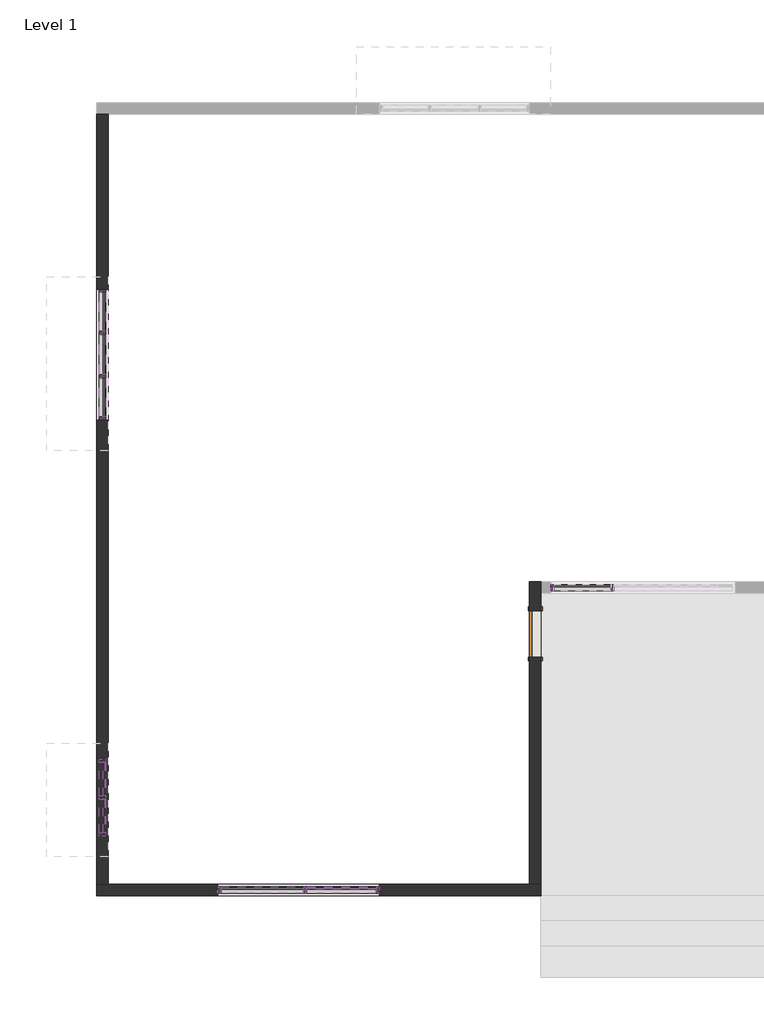
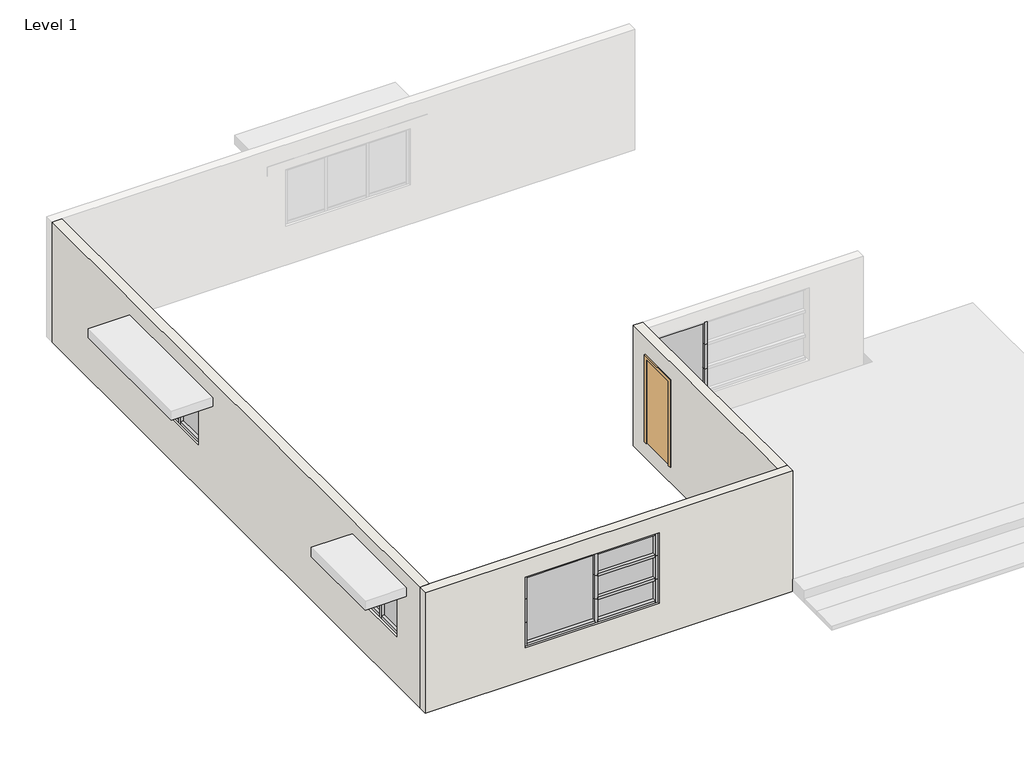
# One storey, part 1 of 2: 39 members, 10 plates, 3 walls, 1 door.
"""IFC4 building model written with IfcOpenShell, lengths in millimetres."""

from ifc_helpers import new_model, si_unit, frame, origin, place, context, project, spatial, polyline, outline, extrude, faceted_brep, transform, mapped, element, save
from components import door_0ca8825f, member_b864958b, member_e6b9f524, member_cfc9b631, member_58197c2e, member_50ab567a, member_249e519d, member_79cc3911, member_4dc7c44e, member_c33c434a, member_8ea09a22, member_05ffdb5f, member_d36207d9, member_46f5bc36, member_488afbc6, member_b07cc7a9, system_panel_glazed_a9ff3cf1, system_panel_glazed_35d8d551, system_panel_glazed_1724a70f, system_panel_glazed_43256be5, system_panel_glazed_960ffd39, system_panel_glazed_d0a3eec4, system_panel_glazed_ba533b82

model = new_model("IFC4")

# Units and contexts
model_context = context("Model", 3, world=origin())
ifc_project = project(units=[si_unit("LENGTHUNIT", "METRE", prefix="MILLI")], contexts=[model_context])

# Site, building, storey
site = spatial("IfcSite", under=ifc_project)
building = spatial("IfcBuilding", under=site)
storey = spatial("IfcBuildingStorey", under=building, Name="Level 1", Elevation=0.0)

# Door
placement = place(None, origin())
door_shape = door_0ca8825f(model_context)
element("IfcDoor", 1, ObjectType="Single-Flush : 36\" x 84\"", at=placement, inside=storey, context=model_context, shape_type="MappedRepresentation", body=[
    mapped(door_shape, transform((-11357.8120831, -6931.6945627, 406.4), x_axis=(0.0, 1.0, 0.0), y_axis=(-1.0, 0.0, 0.0), z_axis=(0.0, 0.0, 1.0))),
])

# Members
member_shape = member_b864958b(model_context)
element("IfcMember", 2, ObjectType="Rectangular Mullion : 2.5\" x 5\" rectangular", at=placement, inside=storey, context=model_context, shape_type="MappedRepresentation", body=[
    mapped(member_shape, transform((-11053.0120831, -6017.2945627, 2097.5096891), x_axis=(-1.0, 0.0, 0.0), y_axis=(0.0, -1.0, 0.0), z_axis=(0.0, 0.0, 1.0))),
])
element("IfcMember", 3, ObjectType="Rectangular Mullion : 2.5\" x 5\" rectangular", at=placement, inside=storey, context=model_context, shape_type="MappedRepresentation", body=[
    mapped(member_shape, transform((-11053.0120831, -6017.2945627, 2710.3034891), x_axis=(-1.0, 0.0, 0.0), y_axis=(0.0, -1.0, 0.0), z_axis=(0.0, 0.0, 1.0))),
])
member_2_shape = member_e6b9f524(model_context)
element("IfcMember", 4, ObjectType="Rectangular Mullion : 2.5\" x 5\" rectangular", at=placement, inside=storey, context=model_context, shape_type="MappedRepresentation", body=[
    mapped(member_2_shape, transform((-10989.5120831, -6017.2945627, 871.9220892), x_axis=(0.0, 0.0, -1.0), y_axis=(0.0, -1.0, 0.0), z_axis=(-1.0, 0.0, 0.0))),
])
element("IfcMember", 5, ObjectType="Rectangular Mullion : 2.5\" x 5\" rectangular", at=placement, inside=storey, context=model_context, shape_type="MappedRepresentation", body=[
    mapped(member_shape, transform((-11053.0120831, -6017.2945627, 1484.7158892), x_axis=(-1.0, 0.0, 0.0), y_axis=(0.0, -1.0, 0.0), z_axis=(0.0, 0.0, 1.0))),
])
member_3_shape = member_cfc9b631(model_context)
element("IfcMember", 6, ObjectType="Rectangular Mullion : 2.5\" x 5\" rectangular", at=placement, inside=storey, context=model_context, shape_type="MappedRepresentation", body=[
    mapped(member_3_shape, transform((-9833.8120831, -6017.2945627, 2097.5096891), x_axis=(1.0, 0.0, 0.0), y_axis=(0.0, -1.0, 0.0), z_axis=(0.0, 0.0, -1.0))),
])
element("IfcMember", 7, ObjectType="Rectangular Mullion : 2.5\" x 5\" rectangular", at=placement, inside=storey, context=model_context, shape_type="MappedRepresentation", body=[
    mapped(member_3_shape, transform((-9833.8120831, -6017.2945627, 1484.7158892), x_axis=(1.0, 0.0, 0.0), y_axis=(0.0, -1.0, 0.0), z_axis=(0.0, 0.0, -1.0))),
])
element("IfcMember", 8, ObjectType="Rectangular Mullion : 2.5\" x 5\" rectangular", at=placement, inside=storey, context=model_context, shape_type="MappedRepresentation", body=[
    mapped(member_3_shape, transform((-9833.8120831, -6017.2945627, 871.9220892), x_axis=(1.0, 0.0, 0.0), y_axis=(0.0, -1.0, 0.0), z_axis=(0.0, 0.0, -1.0))),
])
member_4_shape = member_58197c2e(model_context)
element("IfcMember", 9, ObjectType="Rectangular Mullion : 2.5\" x 5\" rectangular", at=placement, inside=storey, context=model_context, shape_type="MappedRepresentation", body=[
    mapped(member_4_shape, transform((-17644.3120831, -11998.9945627, 2005.3305343), x_axis=(-1.0, 0.0, 0.0), y_axis=(0.0, -1.0, 0.0), z_axis=(0.0, 0.0, 1.0))),
])
element("IfcMember", 10, ObjectType="Rectangular Mullion : 2.5\" x 5\" rectangular", at=placement, inside=storey, context=model_context, shape_type="MappedRepresentation", body=[
    mapped(member_4_shape, transform((-17644.3120831, -11998.9945627, 2600.8541964), x_axis=(-1.0, 0.0, 0.0), y_axis=(0.0, -1.0, 0.0), z_axis=(0.0, 0.0, 1.0))),
])
element("IfcMember", 11, ObjectType="Rectangular Mullion : 2.5\" x 5\" rectangular", at=placement, inside=storey, context=model_context, shape_type="MappedRepresentation", body=[
    mapped(member_4_shape, transform((-17644.3120831, -11998.9945627, 1409.8068722), x_axis=(-1.0, 0.0, 0.0), y_axis=(0.0, -1.0, 0.0), z_axis=(0.0, 0.0, 1.0))),
])
member_5_shape = member_50ab567a(model_context)
element("IfcMember", 12, ObjectType="Rectangular Mullion : 2.5\" x 5\" rectangular", at=placement, inside=storey, context=model_context, shape_type="MappedRepresentation", body=[
    mapped(member_5_shape, transform((-15917.1120831, -11998.9945627, 2005.3305343), x_axis=(1.0, 0.0, 0.0), y_axis=(0.0, -1.0, 0.0), z_axis=(0.0, 0.0, -1.0))),
])
element("IfcMember", 13, ObjectType="Rectangular Mullion : 2.5\" x 5\" rectangular", at=placement, inside=storey, context=model_context, shape_type="MappedRepresentation", body=[
    mapped(member_5_shape, transform((-15917.1120831, -11998.9945627, 1409.8068722), x_axis=(1.0, 0.0, 0.0), y_axis=(0.0, -1.0, 0.0), z_axis=(0.0, 0.0, -1.0))),
])
element("IfcMember", 14, ObjectType="Rectangular Mullion : 2.5\" x 5\" rectangular", at=placement, inside=storey, context=model_context, shape_type="MappedRepresentation", body=[
    mapped(member_5_shape, transform((-15917.1120831, -11998.9945627, 814.2832101), x_axis=(1.0, 0.0, 0.0), y_axis=(0.0, -1.0, 0.0), z_axis=(0.0, 0.0, -1.0))),
])
element("IfcMember", 15, ObjectType="Rectangular Mullion : 2.5\" x 5\" rectangular", at=placement, inside=storey, context=model_context, shape_type="MappedRepresentation", body=[
    mapped(member_4_shape, transform((-14443.9120831, -11998.9945627, 1409.8068722), x_axis=(1.0, 0.0, 0.0), y_axis=(0.0, -1.0, 0.0), z_axis=(0.0, 0.0, -1.0))),
])
element("IfcMember", 16, ObjectType="Rectangular Mullion : 2.5\" x 5\" rectangular", at=placement, inside=storey, context=model_context, shape_type="MappedRepresentation", body=[
    mapped(member_4_shape, transform((-14443.9120831, -11998.9945627, 2005.3305343), x_axis=(1.0, 0.0, 0.0), y_axis=(0.0, -1.0, 0.0), z_axis=(0.0, 0.0, -1.0))),
])
element("IfcMember", 17, ObjectType="Rectangular Mullion : 2.5\" x 5\" rectangular", at=placement, inside=storey, context=model_context, shape_type="MappedRepresentation", body=[
    mapped(member_4_shape, transform((-14443.9120831, -11998.9945627, 814.2832101), x_axis=(1.0, 0.0, 0.0), y_axis=(0.0, -1.0, 0.0), z_axis=(0.0, 0.0, -1.0))),
])
member_6_shape = member_249e519d(model_context)
element("IfcMember", 18, ObjectType="Rectangular Mullion : 2.5\" x 5\" rectangular", at=placement, inside=storey, context=model_context, shape_type="MappedRepresentation", body=[
    mapped(member_6_shape, transform((-15948.8620831, -11998.9945627, 2600.8541964), x_axis=(0.0, 0.0, 1.0), y_axis=(0.0, -1.0, 0.0), z_axis=(1.0, 0.0, 0.0))),
])
element("IfcMember", 19, ObjectType="Rectangular Mullion : 2.5\" x 5\" rectangular", at=placement, inside=storey, context=model_context, shape_type="MappedRepresentation", body=[
    mapped(member_6_shape, transform((-17580.8120831, -11998.9945627, 814.2832101), x_axis=(0.0, 0.0, -1.0), y_axis=(0.0, -1.0, 0.0), z_axis=(-1.0, 0.0, 0.0))),
])
member_7_shape = member_79cc3911(model_context)
element("IfcMember", 20, ObjectType="Rectangular Mullion : 2.5\" x 5\" rectangular", at=placement, inside=storey, context=model_context, shape_type="MappedRepresentation", body=[
    mapped(member_7_shape, transform((-14507.4120831, -11998.9945627, 2600.8541964), x_axis=(0.0, 0.0, 1.0), y_axis=(0.0, -1.0, 0.0), z_axis=(1.0, 0.0, 0.0))),
])
element("IfcMember", 21, ObjectType="Rectangular Mullion : 2.5\" x 5\" rectangular", at=placement, inside=storey, context=model_context, shape_type="MappedRepresentation", body=[
    mapped(member_7_shape, transform((-15885.3620831, -11998.9945627, 814.2832101), x_axis=(0.0, 0.0, -1.0), y_axis=(0.0, -1.0, 0.0), z_axis=(-1.0, 0.0, 0.0))),
])
member_8_shape = member_4dc7c44e(model_context)
element("IfcMember", 22, ObjectType="Rectangular Mullion : 2.5\" x 5\" rectangular", at=placement, inside=storey, context=model_context, shape_type="MappedRepresentation", body=[
    mapped(member_8_shape, transform((-14507.4120831, -11998.9945627, 2005.3305343), x_axis=(0.0, 0.0, 1.0), y_axis=(0.0, -1.0, 0.0), z_axis=(1.0, 0.0, 0.0))),
])
element("IfcMember", 23, ObjectType="Rectangular Mullion : 2.5\" x 5\" rectangular", at=placement, inside=storey, context=model_context, shape_type="MappedRepresentation", body=[
    mapped(member_8_shape, transform((-14507.4120831, -11998.9945627, 1409.8068722), x_axis=(0.0, 0.0, 1.0), y_axis=(0.0, -1.0, 0.0), z_axis=(1.0, 0.0, 0.0))),
])
member_9_shape = member_c33c434a(model_context)
element("IfcMember", 24, ObjectType="Rectangular Mullion : 2.5\" x 5\" rectangular", at=placement, inside=storey, context=model_context, shape_type="MappedRepresentation", body=[
    mapped(member_9_shape, transform((-19930.3120831, -10138.4445627, 2481.0176056), x_axis=(0.0, 0.0, 1.0), y_axis=(-1.0, 0.0, 0.0), z_axis=(0.0, -1.0, 0.0))),
])
element("IfcMember", 25, ObjectType="Rectangular Mullion : 2.5\" x 5\" rectangular", at=placement, inside=storey, context=model_context, shape_type="MappedRepresentation", body=[
    mapped(member_9_shape, transform((-19930.3120831, -10868.6945627, 2481.0176056), x_axis=(0.0, 0.0, 1.0), y_axis=(-1.0, 0.0, 0.0), z_axis=(0.0, -1.0, 0.0))),
])
member_10_shape = member_8ea09a22(model_context)
element("IfcMember", 26, ObjectType="Rectangular Mullion : 2.5\" x 5\" rectangular", at=placement, inside=storey, context=model_context, shape_type="MappedRepresentation", body=[
    mapped(member_10_shape, transform((-19930.3120831, -10170.1945627, 1220.9555927), x_axis=(0.0, -1.0, 0.0), y_axis=(-1.0, 0.0, 0.0), z_axis=(0.0, 0.0, -1.0))),
])
element("IfcMember", 27, ObjectType="Rectangular Mullion : 2.5\" x 5\" rectangular", at=placement, inside=storey, context=model_context, shape_type="MappedRepresentation", body=[
    mapped(member_9_shape, transform((-19930.3120831, -10201.9445627, 1220.9555927), x_axis=(0.0, 0.0, -1.0), y_axis=(-1.0, 0.0, 0.0), z_axis=(0.0, 1.0, 0.0))),
])
element("IfcMember", 28, ObjectType="Rectangular Mullion : 2.5\" x 5\" rectangular", at=placement, inside=storey, context=model_context, shape_type="MappedRepresentation", body=[
    mapped(member_9_shape, transform((-19930.3120831, -9471.6945627, 1220.9555927), x_axis=(0.0, 0.0, -1.0), y_axis=(-1.0, 0.0, 0.0), z_axis=(0.0, 1.0, 0.0))),
])
member_11_shape = member_05ffdb5f(model_context)
element("IfcMember", 29, ObjectType="Rectangular Mullion : 2.5\" x 5\" rectangular", at=placement, inside=storey, context=model_context, shape_type="MappedRepresentation", body=[
    mapped(member_11_shape, transform((-19930.3120831, -9408.1945627, 2481.0176056), x_axis=(0.0, 1.0, 0.0), y_axis=(-1.0, 0.0, 0.0), z_axis=(0.0, 0.0, 1.0))),
])
element("IfcMember", 30, ObjectType="Rectangular Mullion : 2.5\" x 5\" rectangular", at=placement, inside=storey, context=model_context, shape_type="MappedRepresentation", body=[
    mapped(member_11_shape, transform((-19930.3120831, -10932.1945627, 1220.9555927), x_axis=(0.0, -1.0, 0.0), y_axis=(-1.0, 0.0, 0.0), z_axis=(0.0, 0.0, -1.0))),
])
member_12_shape = member_d36207d9(model_context)
element("IfcMember", 31, ObjectType="Rectangular Mullion : 2.5\" x 5\" rectangular", at=placement, inside=storey, context=model_context, shape_type="MappedRepresentation", body=[
    mapped(member_12_shape, transform((-19930.3120831, -1807.2445627, 2422.8588865), x_axis=(0.0, 0.0, 1.0), y_axis=(-1.0, 0.0, 0.0), z_axis=(0.0, -1.0, 0.0))),
])
member_13_shape = member_46f5bc36(model_context)
element("IfcMember", 32, ObjectType="Rectangular Mullion : 2.5\" x 5\" rectangular", at=placement, inside=storey, context=model_context, shape_type="MappedRepresentation", body=[
    mapped(member_13_shape, transform((-19930.3120831, -943.6445627, 2422.8588865), x_axis=(0.0, 0.0, 1.0), y_axis=(-1.0, 0.0, 0.0), z_axis=(0.0, -1.0, 0.0))),
])
element("IfcMember", 33, ObjectType="Rectangular Mullion : 2.5\" x 5\" rectangular", at=placement, inside=storey, context=model_context, shape_type="MappedRepresentation", body=[
    mapped(member_13_shape, transform((-19930.3120831, -2639.0945627, 2422.8588865), x_axis=(0.0, 0.0, 1.0), y_axis=(-1.0, 0.0, 0.0), z_axis=(0.0, -1.0, 0.0))),
])
member_14_shape = member_488afbc6(model_context)
element("IfcMember", 34, ObjectType="Rectangular Mullion : 2.5\" x 5\" rectangular", at=placement, inside=storey, context=model_context, shape_type="MappedRepresentation", body=[
    mapped(member_14_shape, transform((-19930.3120831, -975.3945627, 1079.0309344), x_axis=(0.0, -1.0, 0.0), y_axis=(-1.0, 0.0, 0.0), z_axis=(0.0, 0.0, -1.0))),
])
element("IfcMember", 35, ObjectType="Rectangular Mullion : 2.5\" x 5\" rectangular", at=placement, inside=storey, context=model_context, shape_type="MappedRepresentation", body=[
    mapped(member_14_shape, transform((-19930.3120831, -1838.9945627, 1079.0309344), x_axis=(0.0, -1.0, 0.0), y_axis=(-1.0, 0.0, 0.0), z_axis=(0.0, 0.0, -1.0))),
])
element("IfcMember", 36, ObjectType="Rectangular Mullion : 2.5\" x 5\" rectangular", at=placement, inside=storey, context=model_context, shape_type="MappedRepresentation", body=[
    mapped(member_12_shape, transform((-19930.3120831, -1007.1445627, 1079.0309344), x_axis=(0.0, 0.0, -1.0), y_axis=(-1.0, 0.0, 0.0), z_axis=(0.0, 1.0, 0.0))),
])
element("IfcMember", 37, ObjectType="Rectangular Mullion : 2.5\" x 5\" rectangular", at=placement, inside=storey, context=model_context, shape_type="MappedRepresentation", body=[
    mapped(member_13_shape, transform((-19930.3120831, -1870.7445627, 1079.0309344), x_axis=(0.0, 0.0, -1.0), y_axis=(-1.0, 0.0, 0.0), z_axis=(0.0, 1.0, 0.0))),
])
element("IfcMember", 38, ObjectType="Rectangular Mullion : 2.5\" x 5\" rectangular", at=placement, inside=storey, context=model_context, shape_type="MappedRepresentation", body=[
    mapped(member_13_shape, transform((-19930.3120831, -175.2945627, 1079.0309344), x_axis=(0.0, 0.0, -1.0), y_axis=(-1.0, 0.0, 0.0), z_axis=(0.0, 1.0, 0.0))),
])
member_15_shape = member_b07cc7a9(model_context)
element("IfcMember", 39, ObjectType="Rectangular Mullion : 2.5\" x 5\" rectangular", at=placement, inside=storey, context=model_context, shape_type="MappedRepresentation", body=[
    mapped(member_15_shape, transform((-19930.3120831, -111.7945627, 2422.8588865), x_axis=(0.0, 1.0, 0.0), y_axis=(-1.0, 0.0, 0.0), z_axis=(0.0, 0.0, 1.0))),
])
element("IfcMember", 40, ObjectType="Rectangular Mullion : 2.5\" x 5\" rectangular", at=placement, inside=storey, context=model_context, shape_type="MappedRepresentation", body=[
    mapped(member_15_shape, transform((-19930.3120831, -2702.5945627, 1079.0309344), x_axis=(0.0, -1.0, 0.0), y_axis=(-1.0, 0.0, 0.0), z_axis=(0.0, 0.0, -1.0))),
])

# Plates
system_panel_glazed_shape = system_panel_glazed_a9ff3cf1(model_context)
element("IfcPlate", 41, ObjectType="System Panel : Glazed", at=placement, inside=storey, context=model_context, shape_type="MappedRepresentation", body=[
    mapped(system_panel_glazed_shape, transform((-10427.5370831, -6017.2945627, 935.4220892), x_axis=(1.0, 0.0, 0.0), y_axis=(0.0, 1.0, 0.0), z_axis=(0.0, 0.0, 1.0))),
])
system_panel_glazed_2_shape = system_panel_glazed_35d8d551(model_context)
element("IfcPlate", 42, ObjectType="System Panel : Glazed", at=placement, inside=storey, context=model_context, shape_type="MappedRepresentation", body=[
    mapped(system_panel_glazed_2_shape, transform((-16764.8370831, -11998.9945627, 877.7832101), x_axis=(1.0, 0.0, 0.0), y_axis=(0.0, 1.0, 0.0), z_axis=(0.0, 0.0, 1.0))),
])
system_panel_glazed_3_shape = system_panel_glazed_1724a70f(model_context)
element("IfcPlate", 43, ObjectType="System Panel : Glazed", at=placement, inside=storey, context=model_context, shape_type="MappedRepresentation", body=[
    mapped(system_panel_glazed_3_shape, transform((-15196.3870831, -11998.9945627, 877.7832101), x_axis=(1.0, 0.0, 0.0), y_axis=(0.0, 1.0, 0.0), z_axis=(0.0, 0.0, 1.0))),
])
element("IfcPlate", 44, ObjectType="System Panel : Glazed", at=placement, inside=storey, context=model_context, shape_type="MappedRepresentation", body=[
    mapped(system_panel_glazed_3_shape, transform((-15196.3870831, -11998.9945627, 2037.0805343), x_axis=(1.0, 0.0, 0.0), y_axis=(0.0, 1.0, 0.0), z_axis=(0.0, 0.0, 1.0))),
])
system_panel_glazed_4_shape = system_panel_glazed_43256be5(model_context)
element("IfcPlate", 45, ObjectType="System Panel : Glazed", at=placement, inside=storey, context=model_context, shape_type="MappedRepresentation", body=[
    mapped(system_panel_glazed_4_shape, transform((-15196.3870831, -11998.9945627, 1441.5568722), x_axis=(1.0, 0.0, 0.0), y_axis=(0.0, 1.0, 0.0), z_axis=(0.0, 0.0, 1.0))),
])
system_panel_glazed_5_shape = system_panel_glazed_960ffd39(model_context)
element("IfcPlate", 46, ObjectType="System Panel : Glazed", at=placement, inside=storey, context=model_context, shape_type="MappedRepresentation", body=[
    mapped(system_panel_glazed_5_shape, transform((-19930.3120831, -9805.0695627, 1284.4555927), x_axis=(0.0, -1.0, 0.0), y_axis=(1.0, 0.0, 0.0), z_axis=(0.0, 0.0, 1.0))),
])
element("IfcPlate", 47, ObjectType="System Panel : Glazed", at=placement, inside=storey, context=model_context, shape_type="MappedRepresentation", body=[
    mapped(system_panel_glazed_5_shape, transform((-19930.3120831, -10535.3195627, 1284.4555927), x_axis=(0.0, -1.0, 0.0), y_axis=(1.0, 0.0, 0.0), z_axis=(0.0, 0.0, 1.0))),
])
system_panel_glazed_6_shape = system_panel_glazed_d0a3eec4(model_context)
element("IfcPlate", 48, ObjectType="System Panel : Glazed", at=placement, inside=storey, context=model_context, shape_type="MappedRepresentation", body=[
    mapped(system_panel_glazed_6_shape, transform((-19930.3120831, -559.4695627, 1142.5309344), x_axis=(0.0, -1.0, 0.0), y_axis=(1.0, 0.0, 0.0), z_axis=(0.0, 0.0, 1.0))),
])
element("IfcPlate", 49, ObjectType="System Panel : Glazed", at=placement, inside=storey, context=model_context, shape_type="MappedRepresentation", body=[
    mapped(system_panel_glazed_6_shape, transform((-19930.3120831, -2254.9195627, 1142.5309344), x_axis=(0.0, -1.0, 0.0), y_axis=(1.0, 0.0, 0.0), z_axis=(0.0, 0.0, 1.0))),
])
system_panel_glazed_7_shape = system_panel_glazed_ba533b82(model_context)
element("IfcPlate", 50, ObjectType="System Panel : Glazed", at=placement, inside=storey, context=model_context, shape_type="MappedRepresentation", body=[
    mapped(system_panel_glazed_7_shape, transform((-19930.3120831, -1407.1945627, 1142.5309344), x_axis=(0.0, -1.0, 0.0), y_axis=(1.0, 0.0, 0.0), z_axis=(0.0, 0.0, 1.0))),
])

# Walls
element("IfcWall", 51, ObjectType="9\"", at=placement, inside=storey, context=model_context, shape_type="Brep", body=[
    faceted_brep([(-20044.6120831, -12113.2945627, 0.0), (-11243.5120831, -12113.2945627, 0.0), (-11243.5120831, -12113.2945627, 3048.0), (-20044.6120831, -12113.2945627, 3048.0), (-17644.3120831, -12113.2945627, 814.2832101), (-17644.3120831, -12113.2945627, 2600.8541964), (-14443.9120831, -12113.2945627, 2600.8541964), (-14443.9120831, -12113.2945627, 814.2832101), (-11243.5120831, -11884.6945627, 0.0), (-11472.1120831, -11884.6945627, 0.0), (-19816.0120831, -11884.6945627, 0.0), (-20044.6120831, -11884.6945627, 0.0), (-20044.6120831, -11884.6945627, 3048.0), (-19816.0120831, -11884.6945627, 3048.0), (-11472.1120831, -11884.6945627, 3048.0), (-11243.5120831, -11884.6945627, 3048.0), (-17644.3120831, -11884.6945627, 2600.8541964), (-17644.3120831, -11884.6945627, 814.2832101), (-14443.9120831, -11884.6945627, 814.2832101), (-14443.9120831, -11884.6945627, 2600.8541964)], [[[0, 1, 2, 3], [4, 5, 6, 7]], [[8, 9, 10, 11, 12, 13, 14, 15], [16, 17, 18, 19]], [[1, 0, 11, 10, 9, 8]], [[2, 1, 8, 15]], [[3, 2, 15, 14, 13, 12]], [[0, 3, 12, 11]], [[4, 17, 16, 5]], [[5, 16, 19, 6]], [[6, 19, 18, 7]], [[17, 4, 7, 18]]]),
])
element("IfcWall", 52, ObjectType="9\"", at=placement, inside=storey, context=model_context, shape_type="SweptSolid", body=[
    extrude(outline(polyline([(3355.3054373, 0.0), (-11884.6945627, 0.0), (-11884.6945627, 3048.0), (3355.3054373, 3048.0), (3355.3054373, 0.0)]), holes=[polyline([(-9408.1945627, 1220.9555927), (-9408.1945627, 2481.0176056), (-10932.1945627, 2481.0176056), (-10932.1945627, 1220.9555927), (-9408.1945627, 1220.9555927)]), polyline([(-111.7945627, 1079.0309344), (-111.7945627, 2422.8588865), (-2702.5945627, 2422.8588865), (-2702.5945627, 1079.0309344), (-111.7945627, 1079.0309344)])]), frame((-20044.6120831, 0.0, 0.0), z_axis=(1.0, 0.0, 0.0), x_axis=(0.0, 1.0, 0.0)), (0.0, 0.0, 1.0), 228.6),
])
element("IfcWall", 53, ObjectType="9\"", at=placement, inside=storey, context=model_context, shape_type="Brep", body=[
    faceted_brep([(-11243.5120831, -11884.6945627, 0.0), (-11243.5120831, -6131.5945627, 0.0), (-11243.5120831, -5902.9945627, 0.0), (-11243.5120831, -5902.9945627, 3048.0), (-11243.5120831, -6131.5945627, 3048.0), (-11243.5120831, -11884.6945627, 3048.0), (-11243.5120831, -7388.8945627, 406.4), (-11243.5120831, -7388.8945627, 2540.0), (-11243.5120831, -6474.4945627, 2540.0), (-11243.5120831, -6474.4945627, 406.4), (-11472.1120831, -11884.6945627, 0.0), (-11472.1120831, -11884.6945627, 3048.0), (-11472.1120831, -5902.9945627, 3048.0), (-11472.1120831, -5902.9945627, 0.0), (-11472.1120831, -7388.8945627, 406.4), (-11472.1120831, -6474.4945627, 406.4), (-11472.1120831, -6474.4945627, 2540.0), (-11472.1120831, -7388.8945627, 2540.0)], [[[0, 1, 2, 3, 4, 5], [6, 7, 8, 9]], [[10, 11, 12, 13], [14, 15, 16, 17]], [[2, 1, 0, 10, 13]], [[5, 4, 3, 12, 11]], [[0, 5, 11, 10]], [[3, 2, 13, 12]], [[15, 14, 6, 9]], [[16, 15, 9, 8]], [[17, 16, 8, 7]], [[14, 17, 7, 6]]]),
])

save(model, "model.ifc")

# Revit data of these elements
# Type "Single-Flush : 36\" x 84\""
#   Type Mark = "1"
#   Construction Type Id = "MDOOR"
#   Assembly Code = "C1020"
#   Analytic Construction = "Metal"
#   Thickness = 0' - 2"
#   Heat Transfer Coefficient (U) = 0.651978 BTU/(h·ft²·°F)
#   Height = 7' - 0"
#   Trim Projection Ext = 0' - 1"
#   Trim Projection Int = 0' - 1"
#   Trim Width = 0' - 3"
#   Width = 3' - 0"
#   Define Thermal Properties by = 1
#   Define Thermal Properties by = 1
#   Door Material = Door - Panel
#   Frame Material = Door - Frame
#   Visual Light Transmittance = 0
#   Solar Heat Gain Coefficient = 0
#   Function = (empty or 0)
#   Wall Closure = (empty or 0)
# Type "Rectangular Mullion : 2.5\" x 5\" rectangular"
#   built-in parameter 1007304 = 0.416667 (stored number, unit not read)
#   built-in parameter 1007301 = 0.104167 (stored number, unit not read)
#   built-in parameter 1007300 = 0.104167 (stored number, unit not read)
# Type "System Panel : Glazed"
#   Construction Type Id = "GSP4R"
#   Analytic Construction = "1/8 in Pilkington single glazing"
#   Visual Light Transmittance = 0.9
#   Solar Heat Gain Coefficient = 0.86
#   Heat Transfer Coefficient (U) = 1.18115 BTU/(h·ft²·°F)
#   Define Thermal Properties by = 1
# Type "9\""
#   Assembly Code = "B2010"
#   Layers, outside or top first: 0' - 9" no material (function 1)
# Element 1 (IfcDoor, "Single-Flush : 36\" x 84\"")
#   Phase Created = New Construction
#   Materials on its faces: "Door - Frame", "Door - Panel"
# Elements 2, 3, 4, 5, 6, 7, 8, 9, 10, 11, 12, 13, 14, 15, 16, 17, 18, 19, 20, 21, 22, 23, 24, 25, 26, 27, 28, 29, 30, 31, 32, 33, 34, 35, 36, 37, 38, 39, 40 (IfcMember, "Rectangular Mullion : 2.5\" x 5\" rectangular")
#   Phase Created = New Construction
#   Materials on its faces: "Aluminum"
# Elements 41, 42, 43, 44, 45, 46, 47, 48, 49, 50 (IfcPlate, "System Panel : Glazed")
#   Phase Created = New Construction
#   Materials on its faces: "Glass"
# Elements 51, 52, 53 (IfcWall, "9\"")
#   Top Offset = 0' - 0"
#   Base Offset = 0' - 0"
#   Unconnected Height = 10' - 0"
#   wall height = 10' - 0"
#   Phase Created = New Construction
#   Base Constraint = Level 1
#   Materials on its faces: "Default Wall"
# Materials
#   "Door - Panel": class "Wood", colour RGB 210 159 95, transparency 0, Cost = 0
#   "Door - Frame": colour RGB 118 70 51, transparency 0, Cost = 0
#   "Aluminum": class "Metal", colour RGB 247 247 247, transparency 0, Description = "Aluminum 6061", Cost = 0
#   "Glass": class "Glass", colour RGB 0 128 192, transparency 0.75, Description = "Soda Lime Glass", Cost = 0
#   "Default Wall": colour RGB 128 128 128, transparency 0, Cost = 0
